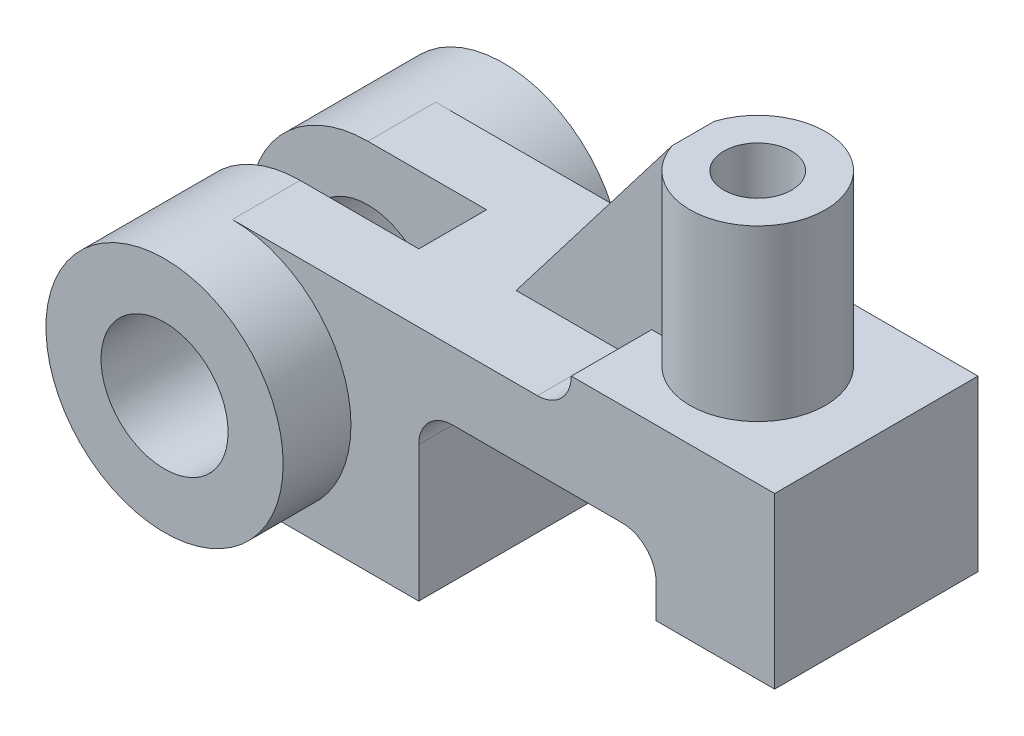
ISO-10303-21;
HEADER;
FILE_DESCRIPTION(('STEP AP214'),'2;1');
FILE_NAME('part.step','',(''),(''),'','','');
FILE_SCHEMA(('AUTOMOTIVE_DESIGN { 1 0 10303 214 1 1 1 1 }'));
ENDSEC;
DATA;
#1=APPLICATION_CONTEXT('core data for automotive mechanical design processes');
#2=APPLICATION_PROTOCOL_DEFINITION('international standard','automotive_design',2000,#1);
#3=PRODUCT_CONTEXT('',#1,'mechanical');
#4=PRODUCT('Part','Part','',(#3));
#5=PRODUCT_RELATED_PRODUCT_CATEGORY('part','',(#4));
#6=PRODUCT_DEFINITION_FORMATION('','',#4);
#7=PRODUCT_DEFINITION_CONTEXT('part definition',#1,'design');
#8=PRODUCT_DEFINITION('design','',#6,#7);
#9=PRODUCT_DEFINITION_SHAPE('','',#8);
#10=(LENGTH_UNIT() NAMED_UNIT(*) SI_UNIT(.MILLI.,.METRE.));
#11=(NAMED_UNIT(*) PLANE_ANGLE_UNIT() SI_UNIT($,.RADIAN.));
#12=(NAMED_UNIT(*) SI_UNIT($,.STERADIAN.) SOLID_ANGLE_UNIT());
#13=UNCERTAINTY_MEASURE_WITH_UNIT(LENGTH_MEASURE(1.E-05),#10,'distance_accuracy_value','');
#14=(GEOMETRIC_REPRESENTATION_CONTEXT(3) GLOBAL_UNCERTAINTY_ASSIGNED_CONTEXT((#13)) GLOBAL_UNIT_ASSIGNED_CONTEXT((#10,
#11,#12)) REPRESENTATION_CONTEXT('',''));
#15=CARTESIAN_POINT('',(0.,0.,0.));
#16=DIRECTION('',(0.,0.,1.));
#17=DIRECTION('',(1.,0.,0.));
#18=AXIS2_PLACEMENT_3D('',#15,#16,#17);
#19=CARTESIAN_POINT('',(0.,28.,0.));
#20=DIRECTION('',(0.,-1.,0.));
#21=DIRECTION('',(0.,0.,-1.));
#22=AXIS2_PLACEMENT_3D('',#19,#20,#21);
#23=PLANE('',#22);
#24=DIRECTION('',(-1.,0.,0.));
#25=VECTOR('',#24,1.);
#26=CARTESIAN_POINT('',(0.,28.,-24.));
#27=LINE('',#26,#25);
#28=CARTESIAN_POINT('',(72.,28.,-24.));
#29=VERTEX_POINT('',#28);
#30=CARTESIAN_POINT('',(0.,28.,-24.));
#31=VERTEX_POINT('',#30);
#32=EDGE_CURVE('E336',#29,#31,#27,.T.);
#33=ORIENTED_EDGE('',*,*,#32,.T.);
#34=DIRECTION('',(0.,0.,1.));
#35=VECTOR('',#34,1.);
#36=CARTESIAN_POINT('',(0.,28.,24.));
#37=LINE('',#36,#35);
#38=CARTESIAN_POINT('',(0.,28.,-8.));
#39=VERTEX_POINT('',#38);
#40=EDGE_CURVE('E326',#31,#39,#37,.T.);
#41=ORIENTED_EDGE('',*,*,#40,.T.);
#42=DIRECTION('',(-1.,0.,0.));
#43=VECTOR('',#42,1.);
#44=CARTESIAN_POINT('',(-32.,28.,-8.));
#45=LINE('',#44,#43);
#46=CARTESIAN_POINT('',(28.,28.,-8.));
#47=VERTEX_POINT('',#46);
#48=EDGE_CURVE('E238',#47,#39,#45,.T.);
#49=ORIENTED_EDGE('',*,*,#48,.F.);
#50=DIRECTION('',(0.,0.,-1.));
#51=VECTOR('',#50,1.);
#52=CARTESIAN_POINT('',(28.,28.,-8.));
#53=LINE('',#52,#51);
#54=CARTESIAN_POINT('',(28.,28.,8.));
#55=VERTEX_POINT('',#54);
#56=EDGE_CURVE('E223',#55,#47,#53,.T.);
#57=ORIENTED_EDGE('',*,*,#56,.F.);
#58=DIRECTION('',(-1.,0.,0.));
#59=VECTOR('',#58,1.);
#60=CARTESIAN_POINT('',(0.,28.,8.));
#61=LINE('',#60,#59);
#62=CARTESIAN_POINT('',(0.,28.,8.));
#63=VERTEX_POINT('',#62);
#64=EDGE_CURVE('E360',#55,#63,#61,.T.);
#65=ORIENTED_EDGE('',*,*,#64,.T.);
#66=CARTESIAN_POINT('',(0.,28.,24.));
#67=VERTEX_POINT('',#66);
#68=EDGE_CURVE('E314',#63,#67,#37,.T.);
#69=ORIENTED_EDGE('',*,*,#68,.T.);
#70=DIRECTION('',(1.,0.,0.));
#71=VECTOR('',#70,1.);
#72=CARTESIAN_POINT('',(0.,28.,24.));
#73=LINE('',#72,#71);
#74=CARTESIAN_POINT('',(72.,28.,24.));
#75=VERTEX_POINT('',#74);
#76=EDGE_CURVE('E331',#67,#75,#73,.T.);
#77=ORIENTED_EDGE('',*,*,#76,.T.);
#78=DIRECTION('',(0.,0.,-1.));
#79=VECTOR('',#78,1.);
#80=CARTESIAN_POINT('',(72.,28.,24.));
#81=LINE('',#80,#79);
#82=CARTESIAN_POINT('',(72.,28.,5.));
#83=VERTEX_POINT('',#82);
#84=EDGE_CURVE('E334',#75,#83,#81,.T.);
#85=ORIENTED_EDGE('',*,*,#84,.T.);
#86=DIRECTION('',(-1.,0.,0.));
#87=VECTOR('',#86,1.);
#88=CARTESIAN_POINT('',(128.002,28.,5.));
#89=LINE('',#88,#87);
#90=CARTESIAN_POINT('',(48.,28.,5.));
#91=VERTEX_POINT('',#90);
#92=EDGE_CURVE('E415',#83,#91,#89,.T.);
#93=ORIENTED_EDGE('',*,*,#92,.T.);
#94=DIRECTION('',(0.,0.,-1.));
#95=VECTOR('',#94,1.);
#96=CARTESIAN_POINT('',(48.,28.,-5.));
#97=LINE('',#96,#95);
#98=CARTESIAN_POINT('',(48.,28.,-5.));
#99=VERTEX_POINT('',#98);
#100=EDGE_CURVE('E195',#91,#99,#97,.T.);
#101=ORIENTED_EDGE('',*,*,#100,.T.);
#102=DIRECTION('',(-1.,0.,0.));
#103=VECTOR('',#102,1.);
#104=CARTESIAN_POINT('',(128.002,28.,-5.));
#105=LINE('',#104,#103);
#106=CARTESIAN_POINT('',(72.,28.,-5.));
#107=VERTEX_POINT('',#106);
#108=EDGE_CURVE('E412',#107,#99,#105,.T.);
#109=ORIENTED_EDGE('',*,*,#108,.F.);
#110=EDGE_CURVE('E333',#107,#29,#81,.T.);
#111=ORIENTED_EDGE('',*,*,#110,.T.);
#112=EDGE_LOOP('',(#33,#41,#49,#57,#65,#69,#77,#85,#93,#101,#109,#111));
#113=FACE_BOUND('',#112,.T.);
#114=ADVANCED_FACE('F44',(#113),#23,.F.);
#115=CARTESIAN_POINT('',(72.,36.,-24.));
#116=DIRECTION('',(0.,1.,0.));
#117=DIRECTION('',(0.,0.,1.));
#118=AXIS2_PLACEMENT_3D('',#115,#116,#117);
#119=PLANE('',#118);
#120=CARTESIAN_POINT('',(100.,36.,0.));
#121=DIRECTION('',(0.,1.,0.));
#122=DIRECTION('',(0.,0.,1.));
#123=AXIS2_PLACEMENT_3D('',#120,#121,#122);
#124=CIRCLE('',#123,16.);
#125=CARTESIAN_POINT('',(84.8013158464293,36.,5.));
#126=VERTEX_POINT('',#125);
#127=CARTESIAN_POINT('',(84.8013158464293,36.,-5.));
#128=VERTEX_POINT('',#127);
#129=EDGE_CURVE('E274',#126,#128,#124,.T.);
#130=ORIENTED_EDGE('',*,*,#129,.F.);
#131=DIRECTION('',(1.,0.,0.));
#132=VECTOR('',#131,1.);
#133=CARTESIAN_POINT('',(128.002,36.,5.));
#134=LINE('',#133,#132);
#135=CARTESIAN_POINT('',(80.,36.,5.));
#136=VERTEX_POINT('',#135);
#137=EDGE_CURVE('E219',#136,#126,#134,.T.);
#138=ORIENTED_EDGE('',*,*,#137,.F.);
#139=DIRECTION('',(0.,0.,1.));
#140=VECTOR('',#139,1.);
#141=CARTESIAN_POINT('',(80.,36.,-40.));
#142=LINE('',#141,#140);
#143=CARTESIAN_POINT('',(80.,36.,24.));
#144=VERTEX_POINT('',#143);
#145=EDGE_CURVE('E358',#144,#136,#142,.F.);
#146=ORIENTED_EDGE('',*,*,#145,.F.);
#147=DIRECTION('',(-1.,0.,0.));
#148=VECTOR('',#147,1.);
#149=CARTESIAN_POINT('',(72.,36.,24.));
#150=LINE('',#149,#148);
#151=CARTESIAN_POINT('',(128.,36.,24.));
#152=VERTEX_POINT('',#151);
#153=EDGE_CURVE('E297',#152,#144,#150,.T.);
#154=ORIENTED_EDGE('',*,*,#153,.F.);
#155=DIRECTION('',(0.,0.,1.));
#156=VECTOR('',#155,1.);
#157=CARTESIAN_POINT('',(128.,36.,-24.));
#158=LINE('',#157,#156);
#159=CARTESIAN_POINT('',(128.,36.,-24.));
#160=VERTEX_POINT('',#159);
#161=EDGE_CURVE('E312',#160,#152,#158,.T.);
#162=ORIENTED_EDGE('',*,*,#161,.F.);
#163=DIRECTION('',(-1.,0.,0.));
#164=VECTOR('',#163,1.);
#165=CARTESIAN_POINT('',(72.,36.,-24.));
#166=LINE('',#165,#164);
#167=CARTESIAN_POINT('',(80.,36.,-24.));
#168=VERTEX_POINT('',#167);
#169=EDGE_CURVE('E303',#160,#168,#166,.T.);
#170=ORIENTED_EDGE('',*,*,#169,.T.);
#171=CARTESIAN_POINT('',(80.,36.,-5.));
#172=VERTEX_POINT('',#171);
#173=EDGE_CURVE('E277',#172,#168,#142,.F.);
#174=ORIENTED_EDGE('',*,*,#173,.F.);
#175=DIRECTION('',(-1.,0.,0.));
#176=VECTOR('',#175,1.);
#177=CARTESIAN_POINT('',(128.002,36.,-5.));
#178=LINE('',#177,#176);
#179=EDGE_CURVE('E229',#128,#172,#178,.T.);
#180=ORIENTED_EDGE('',*,*,#179,.F.);
#181=EDGE_LOOP('',(#130,#138,#146,#154,#162,#170,#174,#180));
#182=FACE_BOUND('',#181,.T.);
#183=ADVANCED_FACE('F406',(#182),#119,.T.);
#184=CARTESIAN_POINT('',(100.,76.,0.));
#185=DIRECTION('',(0.,-1.,0.));
#186=DIRECTION('',(0.,0.,-1.));
#187=AXIS2_PLACEMENT_3D('',#184,#185,#186);
#188=CYLINDRICAL_SURFACE('',#187,16.);
#189=DIRECTION('',(0.,-1.,0.));
#190=VECTOR('',#189,1.);
#191=CARTESIAN_POINT('',(84.8013158464293,76.,5.));
#192=LINE('',#191,#190);
#193=CARTESIAN_POINT('',(84.8013158464293,76.,5.));
#194=VERTEX_POINT('',#193);
#195=EDGE_CURVE('E208',#194,#126,#192,.T.);
#196=ORIENTED_EDGE('',*,*,#195,.T.);
#197=ORIENTED_EDGE('',*,*,#129,.T.);
#198=DIRECTION('',(0.,-1.,0.));
#199=VECTOR('',#198,1.);
#200=CARTESIAN_POINT('',(84.8013158464293,76.,-5.));
#201=LINE('',#200,#199);
#202=CARTESIAN_POINT('',(84.8013158464293,76.,-5.));
#203=VERTEX_POINT('',#202);
#204=EDGE_CURVE('E214',#128,#203,#201,.F.);
#205=ORIENTED_EDGE('',*,*,#204,.T.);
#206=CARTESIAN_POINT('',(100.,76.,0.));
#207=DIRECTION('',(0.,1.,0.));
#208=DIRECTION('',(0.,0.,1.));
#209=AXIS2_PLACEMENT_3D('',#206,#207,#208);
#210=CIRCLE('',#209,16.);
#211=EDGE_CURVE('E202',#194,#203,#210,.T.);
#212=ORIENTED_EDGE('',*,*,#211,.F.);
#213=EDGE_LOOP('',(#196,#197,#205,#212));
#214=FACE_BOUND('',#213,.T.);
#215=ADVANCED_FACE('F206',(#214),#188,.T.);
#216=CARTESIAN_POINT('',(72.,36.,-40.));
#217=DIRECTION('',(0.,0.,1.));
#218=DIRECTION('',(1.,0.,0.));
#219=AXIS2_PLACEMENT_3D('',#216,#217,#218);
#220=CYLINDRICAL_SURFACE('',#219,8.00000000000002);
#221=CARTESIAN_POINT('',(72.,36.,5.));
#222=DIRECTION('',(0.,0.,-1.));
#223=DIRECTION('',(-1.,0.,0.));
#224=AXIS2_PLACEMENT_3D('',#221,#222,#223);
#225=CIRCLE('',#224,8.00000000000002);
#226=EDGE_CURVE('E221',#136,#83,#225,.T.);
#227=ORIENTED_EDGE('',*,*,#226,.T.);
#228=ORIENTED_EDGE('',*,*,#84,.F.);
#229=CARTESIAN_POINT('',(72.,36.,24.));
#230=DIRECTION('',(0.,0.,1.));
#231=DIRECTION('',(-1.,0.,0.));
#232=AXIS2_PLACEMENT_3D('',#229,#230,#231);
#233=CIRCLE('',#232,8.00000000000002);
#234=EDGE_CURVE('E262',#75,#144,#233,.T.);
#235=ORIENTED_EDGE('',*,*,#234,.T.);
#236=ORIENTED_EDGE('',*,*,#145,.T.);
#237=EDGE_LOOP('',(#227,#228,#235,#236));
#238=FACE_BOUND('',#237,.T.);
#239=ADVANCED_FACE('F413',(#238),#220,.F.);
#240=CARTESIAN_POINT('',(72.,36.,-5.));
#241=DIRECTION('',(0.,0.,1.));
#242=DIRECTION('',(0.,-1.,0.));
#243=AXIS2_PLACEMENT_3D('',#240,#241,#242);
#244=CIRCLE('',#243,8.00000000000002);
#245=EDGE_CURVE('E225',#107,#172,#244,.T.);
#246=ORIENTED_EDGE('',*,*,#245,.T.);
#247=ORIENTED_EDGE('',*,*,#173,.T.);
#248=CARTESIAN_POINT('',(72.,36.,-24.));
#249=DIRECTION('',(0.,0.,-1.));
#250=DIRECTION('',(-1.,0.,0.));
#251=AXIS2_PLACEMENT_3D('',#248,#249,#250);
#252=CIRCLE('',#251,8.00000000000002);
#253=EDGE_CURVE('E266',#168,#29,#252,.T.);
#254=ORIENTED_EDGE('',*,*,#253,.T.);
#255=ORIENTED_EDGE('',*,*,#110,.F.);
#256=EDGE_LOOP('',(#246,#247,#254,#255));
#257=FACE_BOUND('',#256,.T.);
#258=ADVANCED_FACE('F424',(#257),#220,.F.);
#259=CARTESIAN_POINT('',(0.,0.,40.));
#260=DIRECTION('',(0.,0.,-1.));
#261=DIRECTION('',(-1.,0.,0.));
#262=AXIS2_PLACEMENT_3D('',#259,#260,#261);
#263=CYLINDRICAL_SURFACE('',#262,28.);
#264=CARTESIAN_POINT('',(0.,0.,-40.));
#265=DIRECTION('',(0.,0.,1.));
#266=DIRECTION('',(1.,0.,0.));
#267=AXIS2_PLACEMENT_3D('',#264,#265,#266);
#268=CIRCLE('',#267,28.);
#269=CARTESIAN_POINT('',(28.,0.,-40.));
#270=VERTEX_POINT('',#269);
#271=EDGE_CURVE('E347',#270,#270,#268,.T.);
#272=ORIENTED_EDGE('',*,*,#271,.T.);
#273=EDGE_LOOP('',(#272));
#274=FACE_BOUND('',#273,.T.);
#275=DIRECTION('',(0.,0.,1.));
#276=VECTOR('',#275,1.);
#277=CARTESIAN_POINT('',(0.,-28.,24.));
#278=LINE('',#277,#276);
#279=CARTESIAN_POINT('',(0.,-28.,-24.));
#280=VERTEX_POINT('',#279);
#281=CARTESIAN_POINT('',(0.,-28.,-8.));
#282=VERTEX_POINT('',#281);
#283=EDGE_CURVE('E319',#280,#282,#278,.T.);
#284=ORIENTED_EDGE('',*,*,#283,.T.);
#285=CARTESIAN_POINT('',(0.,0.,-8.));
#286=DIRECTION('',(0.,0.,-1.));
#287=DIRECTION('',(-1.,0.,0.));
#288=AXIS2_PLACEMENT_3D('',#285,#286,#287);
#289=CIRCLE('',#288,28.);
#290=EDGE_CURVE('E263',#282,#39,#289,.T.);
#291=ORIENTED_EDGE('',*,*,#290,.T.);
#292=ORIENTED_EDGE('',*,*,#40,.F.);
#293=CARTESIAN_POINT('',(0.,0.,-24.));
#294=DIRECTION('',(0.,0.,-1.));
#295=DIRECTION('',(-1.,0.,0.));
#296=AXIS2_PLACEMENT_3D('',#293,#294,#295);
#297=CIRCLE('',#296,28.);
#298=EDGE_CURVE('E345',#31,#280,#297,.T.);
#299=ORIENTED_EDGE('',*,*,#298,.T.);
#300=EDGE_LOOP('',(#284,#291,#292,#299));
#301=FACE_BOUND('',#300,.T.);
#302=ADVANCED_FACE('F433',(#274,#301),#263,.T.);
#303=CARTESIAN_POINT('',(0.,0.,-40.));
#304=DIRECTION('',(0.,0.,1.));
#305=DIRECTION('',(1.,0.,0.));
#306=AXIS2_PLACEMENT_3D('',#303,#304,#305);
#307=CYLINDRICAL_SURFACE('',#306,15.);
#308=CARTESIAN_POINT('',(0.,0.,-8.));
#309=DIRECTION('',(0.,0.,-1.));
#310=DIRECTION('',(-1.,0.,0.));
#311=AXIS2_PLACEMENT_3D('',#308,#309,#310);
#312=CIRCLE('',#311,15.);
#313=CARTESIAN_POINT('',(-15.,0.,-8.));
#314=VERTEX_POINT('',#313);
#315=EDGE_CURVE('E259',#314,#314,#312,.F.);
#316=ORIENTED_EDGE('',*,*,#315,.T.);
#317=EDGE_LOOP('',(#316));
#318=FACE_BOUND('',#317,.T.);
#319=CARTESIAN_POINT('',(0.,0.,-40.));
#320=DIRECTION('',(0.,0.,1.));
#321=DIRECTION('',(1.,0.,0.));
#322=AXIS2_PLACEMENT_3D('',#319,#320,#321);
#323=CIRCLE('',#322,15.);
#324=CARTESIAN_POINT('',(15.,0.,-40.));
#325=VERTEX_POINT('',#324);
#326=EDGE_CURVE('E348',#325,#325,#323,.T.);
#327=ORIENTED_EDGE('',*,*,#326,.F.);
#328=EDGE_LOOP('',(#327));
#329=FACE_BOUND('',#328,.T.);
#330=ADVANCED_FACE('F488',(#318,#329),#307,.F.);
#331=ORIENTED_EDGE('',*,*,#68,.F.);
#332=CARTESIAN_POINT('',(0.,0.,8.));
#333=DIRECTION('',(0.,0.,1.));
#334=DIRECTION('',(1.,0.,0.));
#335=AXIS2_PLACEMENT_3D('',#332,#333,#334);
#336=CIRCLE('',#335,28.);
#337=CARTESIAN_POINT('',(0.,-28.,8.));
#338=VERTEX_POINT('',#337);
#339=EDGE_CURVE('E253',#63,#338,#336,.T.);
#340=ORIENTED_EDGE('',*,*,#339,.T.);
#341=CARTESIAN_POINT('',(0.,-28.,24.));
#342=VERTEX_POINT('',#341);
#343=EDGE_CURVE('E325',#338,#342,#278,.T.);
#344=ORIENTED_EDGE('',*,*,#343,.T.);
#345=CARTESIAN_POINT('',(0.,0.,24.));
#346=DIRECTION('',(0.,0.,1.));
#347=DIRECTION('',(1.,0.,0.));
#348=AXIS2_PLACEMENT_3D('',#345,#346,#347);
#349=CIRCLE('',#348,28.);
#350=EDGE_CURVE('E330',#342,#67,#349,.T.);
#351=ORIENTED_EDGE('',*,*,#350,.T.);
#352=EDGE_LOOP('',(#331,#340,#344,#351));
#353=FACE_BOUND('',#352,.T.);
#354=CARTESIAN_POINT('',(0.,0.,40.));
#355=DIRECTION('',(0.,0.,1.));
#356=DIRECTION('',(1.,0.,0.));
#357=AXIS2_PLACEMENT_3D('',#354,#355,#356);
#358=CIRCLE('',#357,28.);
#359=CARTESIAN_POINT('',(28.,0.,40.));
#360=VERTEX_POINT('',#359);
#361=EDGE_CURVE('E280',#360,#360,#358,.T.);
#362=ORIENTED_EDGE('',*,*,#361,.F.);
#363=EDGE_LOOP('',(#362));
#364=FACE_BOUND('',#363,.T.);
#365=ADVANCED_FACE('F449',(#353,#364),#263,.T.);
#366=CARTESIAN_POINT('',(0.,0.,40.));
#367=DIRECTION('',(0.,0.,1.));
#368=DIRECTION('',(1.,0.,0.));
#369=AXIS2_PLACEMENT_3D('',#366,#367,#368);
#370=PLANE('',#369);
#371=CARTESIAN_POINT('',(0.,0.,40.));
#372=DIRECTION('',(0.,0.,1.));
#373=DIRECTION('',(1.,0.,0.));
#374=AXIS2_PLACEMENT_3D('',#371,#372,#373);
#375=CIRCLE('',#374,15.);
#376=CARTESIAN_POINT('',(15.,0.,40.));
#377=VERTEX_POINT('',#376);
#378=EDGE_CURVE('E343',#377,#377,#375,.T.);
#379=ORIENTED_EDGE('',*,*,#378,.F.);
#380=EDGE_LOOP('',(#379));
#381=FACE_BOUND('',#380,.T.);
#382=ORIENTED_EDGE('',*,*,#361,.T.);
#383=EDGE_LOOP('',(#382));
#384=FACE_BOUND('',#383,.T.);
#385=ADVANCED_FACE('F487',(#381,#384),#370,.T.);
#386=CARTESIAN_POINT('',(0.,0.,-40.));
#387=DIRECTION('',(0.,0.,1.));
#388=DIRECTION('',(1.,0.,0.));
#389=AXIS2_PLACEMENT_3D('',#386,#387,#388);
#390=PLANE('',#389);
#391=ORIENTED_EDGE('',*,*,#326,.T.);
#392=EDGE_LOOP('',(#391));
#393=FACE_BOUND('',#392,.T.);
#394=ORIENTED_EDGE('',*,*,#271,.F.);
#395=EDGE_LOOP('',(#394));
#396=FACE_BOUND('',#395,.T.);
#397=ADVANCED_FACE('F483',(#393,#396),#390,.F.);
#398=CARTESIAN_POINT('',(0.,0.,8.));
#399=DIRECTION('',(0.,0.,1.));
#400=DIRECTION('',(1.,0.,0.));
#401=AXIS2_PLACEMENT_3D('',#398,#399,#400);
#402=CIRCLE('',#401,15.);
#403=CARTESIAN_POINT('',(15.,0.,8.));
#404=VERTEX_POINT('',#403);
#405=EDGE_CURVE('E249',#404,#404,#402,.F.);
#406=ORIENTED_EDGE('',*,*,#405,.T.);
#407=EDGE_LOOP('',(#406));
#408=FACE_BOUND('',#407,.T.);
#409=ORIENTED_EDGE('',*,*,#378,.T.);
#410=EDGE_LOOP('',(#409));
#411=FACE_BOUND('',#410,.T.);
#412=ADVANCED_FACE('F477',(#408,#411),#307,.F.);
#413=CARTESIAN_POINT('',(0.,-28.,-24.));
#414=DIRECTION('',(0.,0.,-1.));
#415=DIRECTION('',(-1.,0.,0.));
#416=AXIS2_PLACEMENT_3D('',#413,#414,#415);
#417=PLANE('',#416);
#418=ORIENTED_EDGE('',*,*,#253,.F.);
#419=ORIENTED_EDGE('',*,*,#169,.F.);
#420=DIRECTION('',(0.,1.,0.));
#421=VECTOR('',#420,1.);
#422=CARTESIAN_POINT('',(128.,-4.,-24.));
#423=LINE('',#422,#421);
#424=CARTESIAN_POINT('',(128.,-4.,-24.));
#425=VERTEX_POINT('',#424);
#426=EDGE_CURVE('E299',#425,#160,#423,.T.);
#427=ORIENTED_EDGE('',*,*,#426,.F.);
#428=DIRECTION('',(1.,0.,0.));
#429=VECTOR('',#428,1.);
#430=CARTESIAN_POINT('',(72.,-4.,-24.));
#431=LINE('',#430,#429);
#432=CARTESIAN_POINT('',(100.,-4.,-24.));
#433=VERTEX_POINT('',#432);
#434=EDGE_CURVE('E300',#433,#425,#431,.T.);
#435=ORIENTED_EDGE('',*,*,#434,.F.);
#436=DIRECTION('',(0.,1.,0.));
#437=VECTOR('',#436,1.);
#438=CARTESIAN_POINT('',(100.,-4.,-24.));
#439=LINE('',#438,#437);
#440=CARTESIAN_POINT('',(100.,4.,-24.));
#441=VERTEX_POINT('',#440);
#442=EDGE_CURVE('E279',#433,#441,#439,.T.);
#443=ORIENTED_EDGE('',*,*,#442,.T.);
#444=CARTESIAN_POINT('',(92.,4.,-24.));
#445=DIRECTION('',(0.,0.,-1.));
#446=DIRECTION('',(-1.,0.,0.));
#447=AXIS2_PLACEMENT_3D('',#444,#445,#446);
#448=CIRCLE('',#447,8.);
#449=CARTESIAN_POINT('',(92.,12.,-24.));
#450=VERTEX_POINT('',#449);
#451=EDGE_CURVE('E11',#441,#450,#448,.F.);
#452=ORIENTED_EDGE('',*,*,#451,.T.);
#453=DIRECTION('',(-1.,0.,0.));
#454=VECTOR('',#453,1.);
#455=CARTESIAN_POINT('',(100.,12.,-24.));
#456=LINE('',#455,#454);
#457=CARTESIAN_POINT('',(52.,12.,-24.));
#458=VERTEX_POINT('',#457);
#459=EDGE_CURVE('E278',#450,#458,#456,.T.);
#460=ORIENTED_EDGE('',*,*,#459,.T.);
#461=CARTESIAN_POINT('',(52.,3.99999999999999,-24.));
#462=DIRECTION('',(0.,0.,-1.));
#463=DIRECTION('',(-1.,0.,0.));
#464=AXIS2_PLACEMENT_3D('',#461,#462,#463);
#465=CIRCLE('',#464,8.);
#466=CARTESIAN_POINT('',(44.,3.99999999999999,-24.));
#467=VERTEX_POINT('',#466);
#468=EDGE_CURVE('E373',#458,#467,#465,.F.);
#469=ORIENTED_EDGE('',*,*,#468,.T.);
#470=DIRECTION('',(0.,-1.,0.));
#471=VECTOR('',#470,1.);
#472=CARTESIAN_POINT('',(44.,12.,-24.));
#473=LINE('',#472,#471);
#474=CARTESIAN_POINT('',(44.,-28.,-24.));
#475=VERTEX_POINT('',#474);
#476=EDGE_CURVE('E282',#467,#475,#473,.T.);
#477=ORIENTED_EDGE('',*,*,#476,.T.);
#478=DIRECTION('',(-1.,0.,0.));
#479=VECTOR('',#478,1.);
#480=CARTESIAN_POINT('',(0.,-28.,-24.));
#481=LINE('',#480,#479);
#482=EDGE_CURVE('E323',#475,#280,#481,.T.);
#483=ORIENTED_EDGE('',*,*,#482,.T.);
#484=ORIENTED_EDGE('',*,*,#298,.F.);
#485=ORIENTED_EDGE('',*,*,#32,.F.);
#486=EDGE_LOOP('',(#418,#419,#427,#435,#443,#452,#460,#469,#477,#483,#484,#485));
#487=FACE_BOUND('',#486,.T.);
#488=ADVANCED_FACE('F377',(#487),#417,.T.);
#489=CARTESIAN_POINT('',(0.,-28.,24.));
#490=DIRECTION('',(0.,0.,1.));
#491=DIRECTION('',(1.,0.,0.));
#492=AXIS2_PLACEMENT_3D('',#489,#490,#491);
#493=PLANE('',#492);
#494=ORIENTED_EDGE('',*,*,#234,.F.);
#495=ORIENTED_EDGE('',*,*,#76,.F.);
#496=ORIENTED_EDGE('',*,*,#350,.F.);
#497=DIRECTION('',(1.,0.,0.));
#498=VECTOR('',#497,1.);
#499=CARTESIAN_POINT('',(0.,-28.,24.));
#500=LINE('',#499,#498);
#501=CARTESIAN_POINT('',(44.,-28.,24.));
#502=VERTEX_POINT('',#501);
#503=EDGE_CURVE('E322',#342,#502,#500,.T.);
#504=ORIENTED_EDGE('',*,*,#503,.T.);
#505=DIRECTION('',(0.,-1.,0.));
#506=VECTOR('',#505,1.);
#507=CARTESIAN_POINT('',(44.,12.,24.));
#508=LINE('',#507,#506);
#509=CARTESIAN_POINT('',(44.,3.99999999999999,24.));
#510=VERTEX_POINT('',#509);
#511=EDGE_CURVE('E283',#510,#502,#508,.T.);
#512=ORIENTED_EDGE('',*,*,#511,.F.);
#513=CARTESIAN_POINT('',(52.,3.99999999999999,24.));
#514=DIRECTION('',(0.,0.,1.));
#515=DIRECTION('',(1.,0.,0.));
#516=AXIS2_PLACEMENT_3D('',#513,#514,#515);
#517=CIRCLE('',#516,8.);
#518=CARTESIAN_POINT('',(52.,12.,24.));
#519=VERTEX_POINT('',#518);
#520=EDGE_CURVE('E371',#510,#519,#517,.F.);
#521=ORIENTED_EDGE('',*,*,#520,.T.);
#522=DIRECTION('',(-1.,0.,0.));
#523=VECTOR('',#522,1.);
#524=CARTESIAN_POINT('',(100.,12.,24.));
#525=LINE('',#524,#523);
#526=CARTESIAN_POINT('',(92.,12.,24.));
#527=VERTEX_POINT('',#526);
#528=EDGE_CURVE('E287',#527,#519,#525,.T.);
#529=ORIENTED_EDGE('',*,*,#528,.F.);
#530=CARTESIAN_POINT('',(92.,4.,24.));
#531=DIRECTION('',(0.,0.,1.));
#532=DIRECTION('',(1.,0.,0.));
#533=AXIS2_PLACEMENT_3D('',#530,#531,#532);
#534=CIRCLE('',#533,8.);
#535=CARTESIAN_POINT('',(100.,4.,24.));
#536=VERTEX_POINT('',#535);
#537=EDGE_CURVE('E52',#527,#536,#534,.F.);
#538=ORIENTED_EDGE('',*,*,#537,.T.);
#539=DIRECTION('',(0.,1.,0.));
#540=VECTOR('',#539,1.);
#541=CARTESIAN_POINT('',(100.,-4.,24.));
#542=LINE('',#541,#540);
#543=CARTESIAN_POINT('',(100.,-4.,24.));
#544=VERTEX_POINT('',#543);
#545=EDGE_CURVE('E211',#544,#536,#542,.T.);
#546=ORIENTED_EDGE('',*,*,#545,.F.);
#547=DIRECTION('',(1.,0.,0.));
#548=VECTOR('',#547,1.);
#549=CARTESIAN_POINT('',(72.,-4.,24.));
#550=LINE('',#549,#548);
#551=CARTESIAN_POINT('',(128.,-4.,24.));
#552=VERTEX_POINT('',#551);
#553=EDGE_CURVE('E294',#544,#552,#550,.T.);
#554=ORIENTED_EDGE('',*,*,#553,.T.);
#555=DIRECTION('',(0.,1.,0.));
#556=VECTOR('',#555,1.);
#557=CARTESIAN_POINT('',(128.,-4.,24.));
#558=LINE('',#557,#556);
#559=EDGE_CURVE('E308',#552,#152,#558,.T.);
#560=ORIENTED_EDGE('',*,*,#559,.T.);
#561=ORIENTED_EDGE('',*,*,#153,.T.);
#562=EDGE_LOOP('',(#494,#495,#496,#504,#512,#521,#529,#538,#546,#554,#560,#561));
#563=FACE_BOUND('',#562,.T.);
#564=ADVANCED_FACE('F388',(#563),#493,.T.);
#565=CARTESIAN_POINT('',(0.,-28.,0.));
#566=DIRECTION('',(0.,-1.,0.));
#567=DIRECTION('',(0.,0.,-1.));
#568=AXIS2_PLACEMENT_3D('',#565,#566,#567);
#569=PLANE('',#568);
#570=DIRECTION('',(-1.,0.,0.));
#571=VECTOR('',#570,1.);
#572=CARTESIAN_POINT('',(-32.,-28.,-8.));
#573=LINE('',#572,#571);
#574=CARTESIAN_POINT('',(28.,-28.,-8.));
#575=VERTEX_POINT('',#574);
#576=EDGE_CURVE('E241',#575,#282,#573,.T.);
#577=ORIENTED_EDGE('',*,*,#576,.T.);
#578=ORIENTED_EDGE('',*,*,#283,.F.);
#579=ORIENTED_EDGE('',*,*,#482,.F.);
#580=DIRECTION('',(0.,0.,1.));
#581=VECTOR('',#580,1.);
#582=CARTESIAN_POINT('',(44.,-28.,-24.));
#583=LINE('',#582,#581);
#584=EDGE_CURVE('E292',#475,#502,#583,.T.);
#585=ORIENTED_EDGE('',*,*,#584,.T.);
#586=ORIENTED_EDGE('',*,*,#503,.F.);
#587=ORIENTED_EDGE('',*,*,#343,.F.);
#588=DIRECTION('',(1.,0.,0.));
#589=VECTOR('',#588,1.);
#590=CARTESIAN_POINT('',(-32.,-28.,8.));
#591=LINE('',#590,#589);
#592=CARTESIAN_POINT('',(28.,-28.,8.));
#593=VERTEX_POINT('',#592);
#594=EDGE_CURVE('E234',#338,#593,#591,.T.);
#595=ORIENTED_EDGE('',*,*,#594,.T.);
#596=DIRECTION('',(0.,0.,-1.));
#597=VECTOR('',#596,1.);
#598=CARTESIAN_POINT('',(28.,-28.,-8.));
#599=LINE('',#598,#597);
#600=EDGE_CURVE('E240',#593,#575,#599,.T.);
#601=ORIENTED_EDGE('',*,*,#600,.T.);
#602=EDGE_LOOP('',(#577,#578,#579,#585,#586,#587,#595,#601));
#603=FACE_BOUND('',#602,.T.);
#604=ADVANCED_FACE('F437',(#603),#569,.T.);
#605=CARTESIAN_POINT('',(128.,-4.,-24.));
#606=DIRECTION('',(1.,0.,0.));
#607=DIRECTION('',(0.,0.,-1.));
#608=AXIS2_PLACEMENT_3D('',#605,#606,#607);
#609=PLANE('',#608);
#610=ORIENTED_EDGE('',*,*,#559,.F.);
#611=DIRECTION('',(0.,0.,1.));
#612=VECTOR('',#611,1.);
#613=CARTESIAN_POINT('',(128.,-4.,-24.));
#614=LINE('',#613,#612);
#615=EDGE_CURVE('E306',#425,#552,#614,.T.);
#616=ORIENTED_EDGE('',*,*,#615,.F.);
#617=ORIENTED_EDGE('',*,*,#426,.T.);
#618=ORIENTED_EDGE('',*,*,#161,.T.);
#619=EDGE_LOOP('',(#610,#616,#617,#618));
#620=FACE_BOUND('',#619,.T.);
#621=ADVANCED_FACE('F649',(#620),#609,.T.);
#622=CARTESIAN_POINT('',(72.,-4.,-24.));
#623=DIRECTION('',(0.,-1.,0.));
#624=DIRECTION('',(0.,0.,-1.));
#625=AXIS2_PLACEMENT_3D('',#622,#623,#624);
#626=PLANE('',#625);
#627=DIRECTION('',(0.,0.,1.));
#628=VECTOR('',#627,1.);
#629=CARTESIAN_POINT('',(100.,-4.,-24.));
#630=LINE('',#629,#628);
#631=EDGE_CURVE('E286',#433,#544,#630,.T.);
#632=ORIENTED_EDGE('',*,*,#631,.F.);
#633=ORIENTED_EDGE('',*,*,#434,.T.);
#634=ORIENTED_EDGE('',*,*,#615,.T.);
#635=ORIENTED_EDGE('',*,*,#553,.F.);
#636=EDGE_LOOP('',(#632,#633,#634,#635));
#637=FACE_BOUND('',#636,.T.);
#638=ADVANCED_FACE('F405',(#637),#626,.T.);
#639=CARTESIAN_POINT('',(44.,12.,-24.));
#640=DIRECTION('',(-1.,0.,0.));
#641=DIRECTION('',(0.,-1.,0.));
#642=AXIS2_PLACEMENT_3D('',#639,#640,#641);
#643=PLANE('',#642);
#644=ORIENTED_EDGE('',*,*,#476,.F.);
#645=DIRECTION('',(0.,0.,1.));
#646=VECTOR('',#645,1.);
#647=CARTESIAN_POINT('',(44.,3.99999999999999,24.));
#648=LINE('',#647,#646);
#649=EDGE_CURVE('E365',#467,#510,#648,.T.);
#650=ORIENTED_EDGE('',*,*,#649,.T.);
#651=ORIENTED_EDGE('',*,*,#511,.T.);
#652=ORIENTED_EDGE('',*,*,#584,.F.);
#653=EDGE_LOOP('',(#644,#650,#651,#652));
#654=FACE_BOUND('',#653,.T.);
#655=ADVANCED_FACE('F383',(#654),#643,.F.);
#656=CARTESIAN_POINT('',(100.,12.,-24.));
#657=DIRECTION('',(0.,1.,0.));
#658=DIRECTION('',(-1.,0.,0.));
#659=AXIS2_PLACEMENT_3D('',#656,#657,#658);
#660=PLANE('',#659);
#661=ORIENTED_EDGE('',*,*,#528,.T.);
#662=DIRECTION('',(0.,0.,1.));
#663=VECTOR('',#662,1.);
#664=CARTESIAN_POINT('',(52.,12.,-24.));
#665=LINE('',#664,#663);
#666=EDGE_CURVE('E368',#519,#458,#665,.F.);
#667=ORIENTED_EDGE('',*,*,#666,.T.);
#668=ORIENTED_EDGE('',*,*,#459,.F.);
#669=DIRECTION('',(0.,0.,1.));
#670=VECTOR('',#669,1.);
#671=CARTESIAN_POINT('',(92.,12.,24.));
#672=LINE('',#671,#670);
#673=EDGE_CURVE('E362',#450,#527,#672,.T.);
#674=ORIENTED_EDGE('',*,*,#673,.T.);
#675=EDGE_LOOP('',(#661,#667,#668,#674));
#676=FACE_BOUND('',#675,.T.);
#677=ADVANCED_FACE('F395',(#676),#660,.F.);
#678=CARTESIAN_POINT('',(100.,-4.,-24.));
#679=DIRECTION('',(1.,0.,0.));
#680=DIRECTION('',(0.,0.,-1.));
#681=AXIS2_PLACEMENT_3D('',#678,#679,#680);
#682=PLANE('',#681);
#683=ORIENTED_EDGE('',*,*,#545,.T.);
#684=DIRECTION('',(0.,0.,1.));
#685=VECTOR('',#684,1.);
#686=CARTESIAN_POINT('',(100.,4.,-24.));
#687=LINE('',#686,#685);
#688=EDGE_CURVE('E58',#536,#441,#687,.F.);
#689=ORIENTED_EDGE('',*,*,#688,.T.);
#690=ORIENTED_EDGE('',*,*,#442,.F.);
#691=ORIENTED_EDGE('',*,*,#631,.T.);
#692=EDGE_LOOP('',(#683,#689,#690,#691));
#693=FACE_BOUND('',#692,.T.);
#694=ADVANCED_FACE('F398',(#693),#682,.F.);
#695=CARTESIAN_POINT('',(100.,76.,0.));
#696=DIRECTION('',(0.,1.,0.));
#697=DIRECTION('',(0.,0.,1.));
#698=AXIS2_PLACEMENT_3D('',#695,#696,#697);
#699=PLANE('',#698);
#700=DIRECTION('',(0.,0.,-1.));
#701=VECTOR('',#700,1.);
#702=CARTESIAN_POINT('',(84.8013158464293,76.,259.803846124818));
#703=LINE('',#702,#701);
#704=EDGE_CURVE('E186',#194,#203,#703,.T.);
#705=ORIENTED_EDGE('',*,*,#704,.F.);
#706=ORIENTED_EDGE('',*,*,#211,.T.);
#707=EDGE_LOOP('',(#705,#706));
#708=FACE_BOUND('',#707,.T.);
#709=CARTESIAN_POINT('',(100.,76.,0.));
#710=DIRECTION('',(0.,1.,0.));
#711=DIRECTION('',(0.,0.,1.));
#712=AXIS2_PLACEMENT_3D('',#709,#710,#711);
#713=CIRCLE('',#712,8.00000000000001);
#714=CARTESIAN_POINT('',(100.,76.,8.00000000000001));
#715=VERTEX_POINT('',#714);
#716=EDGE_CURVE('E268',#715,#715,#713,.T.);
#717=ORIENTED_EDGE('',*,*,#716,.F.);
#718=EDGE_LOOP('',(#717));
#719=FACE_BOUND('',#718,.T.);
#720=ADVANCED_FACE('F201',(#708,#719),#699,.T.);
#721=CARTESIAN_POINT('',(100.,36.,0.));
#722=DIRECTION('',(0.,1.,0.));
#723=DIRECTION('',(0.,0.,1.));
#724=AXIS2_PLACEMENT_3D('',#721,#722,#723);
#725=CYLINDRICAL_SURFACE('',#724,8.00000000000001);
#726=CARTESIAN_POINT('',(100.,36.,0.));
#727=DIRECTION('',(0.,1.,0.));
#728=DIRECTION('',(0.,0.,1.));
#729=AXIS2_PLACEMENT_3D('',#726,#727,#728);
#730=CIRCLE('',#729,8.00000000000001);
#731=CARTESIAN_POINT('',(100.,36.,8.00000000000001));
#732=VERTEX_POINT('',#731);
#733=EDGE_CURVE('E213',#732,#732,#730,.T.);
#734=ORIENTED_EDGE('',*,*,#733,.F.);
#735=EDGE_LOOP('',(#734));
#736=FACE_BOUND('',#735,.T.);
#737=ORIENTED_EDGE('',*,*,#716,.T.);
#738=EDGE_LOOP('',(#737));
#739=FACE_BOUND('',#738,.T.);
#740=ADVANCED_FACE('F601',(#736,#739),#725,.F.);
#741=CARTESIAN_POINT('',(100.,36.,0.));
#742=DIRECTION('',(0.,1.,0.));
#743=DIRECTION('',(0.,0.,1.));
#744=AXIS2_PLACEMENT_3D('',#741,#742,#743);
#745=PLANE('',#744);
#746=ORIENTED_EDGE('',*,*,#733,.T.);
#747=EDGE_LOOP('',(#746));
#748=FACE_BOUND('',#747,.T.);
#749=ADVANCED_FACE('F461',(#748),#745,.T.);
#750=CARTESIAN_POINT('',(-32.,-28.,-8.));
#751=DIRECTION('',(0.,0.,-1.));
#752=DIRECTION('',(-1.,0.,0.));
#753=AXIS2_PLACEMENT_3D('',#750,#751,#752);
#754=PLANE('',#753);
#755=ORIENTED_EDGE('',*,*,#315,.F.);
#756=EDGE_LOOP('',(#755));
#757=FACE_BOUND('',#756,.T.);
#758=ORIENTED_EDGE('',*,*,#576,.F.);
#759=DIRECTION('',(0.,1.,0.));
#760=VECTOR('',#759,1.);
#761=CARTESIAN_POINT('',(28.,-28.,-8.));
#762=LINE('',#761,#760);
#763=EDGE_CURVE('E247',#575,#47,#762,.T.);
#764=ORIENTED_EDGE('',*,*,#763,.T.);
#765=ORIENTED_EDGE('',*,*,#48,.T.);
#766=ORIENTED_EDGE('',*,*,#290,.F.);
#767=EDGE_LOOP('',(#758,#764,#765,#766));
#768=FACE_BOUND('',#767,.T.);
#769=ADVANCED_FACE('F440',(#757,#768),#754,.F.);
#770=CARTESIAN_POINT('',(-32.,-28.,8.));
#771=DIRECTION('',(0.,0.,1.));
#772=DIRECTION('',(1.,0.,0.));
#773=AXIS2_PLACEMENT_3D('',#770,#771,#772);
#774=PLANE('',#773);
#775=ORIENTED_EDGE('',*,*,#405,.F.);
#776=EDGE_LOOP('',(#775));
#777=FACE_BOUND('',#776,.T.);
#778=ORIENTED_EDGE('',*,*,#64,.F.);
#779=DIRECTION('',(0.,1.,0.));
#780=VECTOR('',#779,1.);
#781=CARTESIAN_POINT('',(28.,-28.,8.));
#782=LINE('',#781,#780);
#783=EDGE_CURVE('E242',#593,#55,#782,.T.);
#784=ORIENTED_EDGE('',*,*,#783,.F.);
#785=ORIENTED_EDGE('',*,*,#594,.F.);
#786=ORIENTED_EDGE('',*,*,#339,.F.);
#787=EDGE_LOOP('',(#778,#784,#785,#786));
#788=FACE_BOUND('',#787,.T.);
#789=ADVANCED_FACE('F455',(#777,#788),#774,.F.);
#790=CARTESIAN_POINT('',(28.,-28.,-8.));
#791=DIRECTION('',(1.,0.,0.));
#792=DIRECTION('',(0.,0.,-1.));
#793=AXIS2_PLACEMENT_3D('',#790,#791,#792);
#794=PLANE('',#793);
#795=ORIENTED_EDGE('',*,*,#56,.T.);
#796=ORIENTED_EDGE('',*,*,#763,.F.);
#797=ORIENTED_EDGE('',*,*,#600,.F.);
#798=ORIENTED_EDGE('',*,*,#783,.T.);
#799=EDGE_LOOP('',(#795,#796,#797,#798));
#800=FACE_BOUND('',#799,.T.);
#801=ADVANCED_FACE('F442',(#800),#794,.F.);
#802=CARTESIAN_POINT('',(128.002,28.,5.));
#803=DIRECTION('',(0.,0.,-1.));
#804=DIRECTION('',(-1.,0.,0.));
#805=AXIS2_PLACEMENT_3D('',#802,#803,#804);
#806=PLANE('',#805);
#807=ORIENTED_EDGE('',*,*,#195,.F.);
#808=DIRECTION('',(0.6084452452408,0.793595856556637,0.));
#809=VECTOR('',#808,1.);
#810=CARTESIAN_POINT('',(84.8013158464293,76.,5.));
#811=LINE('',#810,#809);
#812=EDGE_CURVE('E187',#91,#194,#811,.T.);
#813=ORIENTED_EDGE('',*,*,#812,.F.);
#814=ORIENTED_EDGE('',*,*,#92,.F.);
#815=ORIENTED_EDGE('',*,*,#226,.F.);
#816=ORIENTED_EDGE('',*,*,#137,.T.);
#817=EDGE_LOOP('',(#807,#813,#814,#815,#816));
#818=FACE_BOUND('',#817,.T.);
#819=ADVANCED_FACE('F216',(#818),#806,.F.);
#820=CARTESIAN_POINT('',(128.002,28.,-5.));
#821=DIRECTION('',(0.,0.,1.));
#822=DIRECTION('',(0.,-1.,0.));
#823=AXIS2_PLACEMENT_3D('',#820,#821,#822);
#824=PLANE('',#823);
#825=ORIENTED_EDGE('',*,*,#108,.T.);
#826=DIRECTION('',(0.6084452452408,0.793595856556637,0.));
#827=VECTOR('',#826,1.);
#828=CARTESIAN_POINT('',(77.6171897277239,66.629735764426,-5.));
#829=LINE('',#828,#827);
#830=EDGE_CURVE('E203',#99,#203,#829,.T.);
#831=ORIENTED_EDGE('',*,*,#830,.T.);
#832=ORIENTED_EDGE('',*,*,#204,.F.);
#833=ORIENTED_EDGE('',*,*,#179,.T.);
#834=ORIENTED_EDGE('',*,*,#245,.F.);
#835=EDGE_LOOP('',(#825,#831,#832,#833,#834));
#836=FACE_BOUND('',#835,.T.);
#837=ADVANCED_FACE('F419',(#836),#824,.F.);
#838=CARTESIAN_POINT('',(84.8013158464293,76.,259.803846124818));
#839=DIRECTION('',(0.793595856556637,-0.6084452452408,0.));
#840=DIRECTION('',(0.6084452452408,0.793595856556637,0.));
#841=AXIS2_PLACEMENT_3D('',#838,#839,#840);
#842=PLANE('',#841);
#843=ORIENTED_EDGE('',*,*,#830,.F.);
#844=ORIENTED_EDGE('',*,*,#100,.F.);
#845=ORIENTED_EDGE('',*,*,#812,.T.);
#846=ORIENTED_EDGE('',*,*,#704,.T.);
#847=EDGE_LOOP('',(#843,#844,#845,#846));
#848=FACE_BOUND('',#847,.T.);
#849=ADVANCED_FACE('F189',(#848),#842,.F.);
#850=CARTESIAN_POINT('',(52.,3.99999999999999,-24.));
#851=DIRECTION('',(0.,0.,-1.));
#852=DIRECTION('',(-1.,0.,0.));
#853=AXIS2_PLACEMENT_3D('',#850,#851,#852);
#854=CYLINDRICAL_SURFACE('',#853,8.);
#855=ORIENTED_EDGE('',*,*,#468,.F.);
#856=ORIENTED_EDGE('',*,*,#666,.F.);
#857=ORIENTED_EDGE('',*,*,#520,.F.);
#858=ORIENTED_EDGE('',*,*,#649,.F.);
#859=EDGE_LOOP('',(#855,#856,#857,#858));
#860=FACE_BOUND('',#859,.T.);
#861=ADVANCED_FACE('F389',(#860),#854,.F.);
#862=CARTESIAN_POINT('',(92.,4.,-24.));
#863=DIRECTION('',(0.,0.,-1.));
#864=DIRECTION('',(-1.,0.,0.));
#865=AXIS2_PLACEMENT_3D('',#862,#863,#864);
#866=CYLINDRICAL_SURFACE('',#865,8.);
#867=ORIENTED_EDGE('',*,*,#451,.F.);
#868=ORIENTED_EDGE('',*,*,#688,.F.);
#869=ORIENTED_EDGE('',*,*,#537,.F.);
#870=ORIENTED_EDGE('',*,*,#673,.F.);
#871=EDGE_LOOP('',(#867,#868,#869,#870));
#872=FACE_BOUND('',#871,.T.);
#873=ADVANCED_FACE('F50',(#872),#866,.F.);
#874=CLOSED_SHELL('',(#114,#183,#215,#239,#258,#302,#330,#365,#385,#397,#412,#488,#564,#604,
#621,#638,#655,#677,#694,#720,#740,#749,#769,#789,#801,#819,#837,#849,#861,#873));
#875=MANIFOLD_SOLID_BREP('B2',#874);
#876=ADVANCED_BREP_SHAPE_REPRESENTATION('',(#18,#875),#14);
#877=SHAPE_DEFINITION_REPRESENTATION(#9,#876);
ENDSEC;
END-ISO-10303-21;
